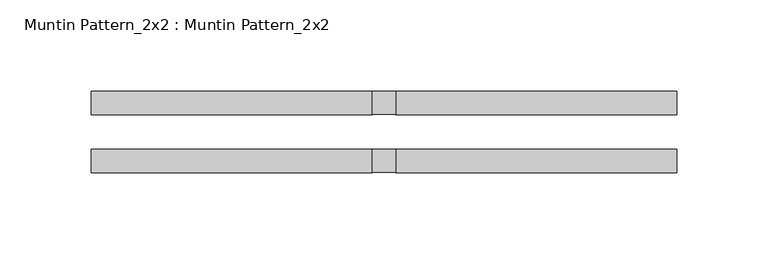
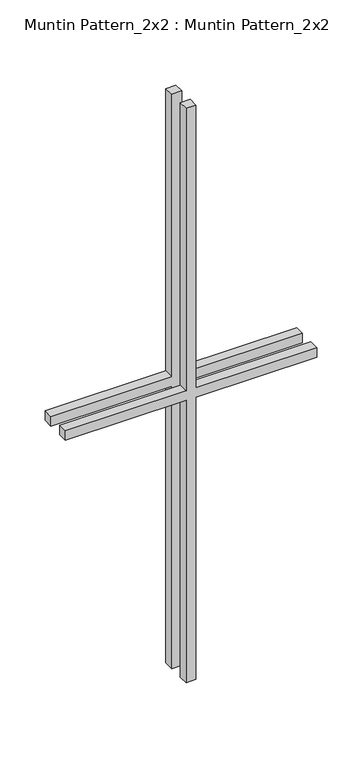
"""IFC4 building model written with IfcOpenShell, lengths in millimetres: proxy geometry, Muntin Pattern_2x2 : Muntin Pattern_2x2."""

from ifc_helpers import new_model, si_unit, frame, origin, place, context, project, spatial, polyline, outline, extrude, source, transform, mapped, element, save


def muntin_pattern_2x2_muntin_pattern_2x2_d1c6e638(model_context):
    return source(origin(), model_context, "Body", "SweptSolid", [
        extrude(outline(polyline([(393.7, -6.35), (393.7, -160.3375), (381.0, -160.3375), (381.0, -6.35), (0.0, -6.35), (0.0, 6.35), (381.0, 6.35), (381.0, 160.3375), (393.7, 160.3375), (393.7, 6.35), (774.7, 6.35), (774.7, -6.35), (393.7, -6.35)])), frame((0.0, 9.525, 0.0), z_axis=(0.0, 1.0, 0.0), x_axis=(0.0, 0.0, 1.0)), (0.0, 0.0, 1.0), 12.7),
        extrude(outline(polyline([(393.7, -6.35), (393.7, -160.3375), (381.0, -160.3375), (381.0, -6.35), (0.0, -6.35), (0.0, 6.35), (381.0, 6.35), (381.0, 160.3375), (393.7, 160.3375), (393.7, 6.35), (774.7, 6.35), (774.7, -6.35), (393.7, -6.35)])), frame((0.0, -22.225, 0.0), z_axis=(0.0, 1.0, 0.0), x_axis=(0.0, 0.0, 1.0)), (0.0, 0.0, 1.0), 12.7),
    ])


if __name__ == "__main__":
    model = new_model("IFC4")
    model_context = context("Model", 3, world=origin())
    ifc_project = project(units=[si_unit("LENGTHUNIT", "METRE", prefix="MILLI")], contexts=[model_context])
    site = spatial("IfcSite", under=ifc_project)
    building = spatial("IfcBuilding", under=site)
    placement = place(None, origin())
    muntin_pattern_2x2_muntin_pattern_2x2_shape = muntin_pattern_2x2_muntin_pattern_2x2_d1c6e638(model_context)
    element("IfcBuildingElementProxy", 1, Name="Muntin Pattern_2x2 : Muntin Pattern_2x2", ObjectType="Muntin Pattern_2x2 : Muntin Pattern_2x2", at=placement, inside=building, context=model_context, shape_type="MappedRepresentation", body=[
        mapped(muntin_pattern_2x2_muntin_pattern_2x2_shape, transform((0.0, 0.0, 0.0), x_axis=(1.0, 0.0, 0.0), y_axis=(0.0, 1.0, 0.0), z_axis=(0.0, 0.0, 1.0))),
    ])
    save(model, "model.ifc")

# Revit data of these elements
# Type "Muntin Pattern_2x2 : Muntin Pattern_2x2"
#   Width [instance default] = 4' - 0"
#   Thickness = 0' - 0 1/2"
#   Height [instance default] = 4' - 0"
#   Distance = 0' - 0 3/4"
#   Interior Material [instance default] = none
#   Exterior Material [instance default] = none
#   Default Elevation = 0
# Element 1 (IfcBuildingElementProxy, "Muntin Pattern_2x2 : Muntin Pattern_2x2")
#   Width = 1' - 0 5/8"
#   Height = 2' - 6 1/2"
#   Interior Material = Wood - Stained
#   Exterior Material = Clad - White
#   Materials on its faces: "Clad - White", "Wood - Stained"
# Materials
#   "Clad - White": class "Wood", colour RGB 242 242 238, transparency 0, Cost = 0
#   "Wood - Stained": class "Wood", colour RGB 224 178 126, transparency 0, Cost = 0
